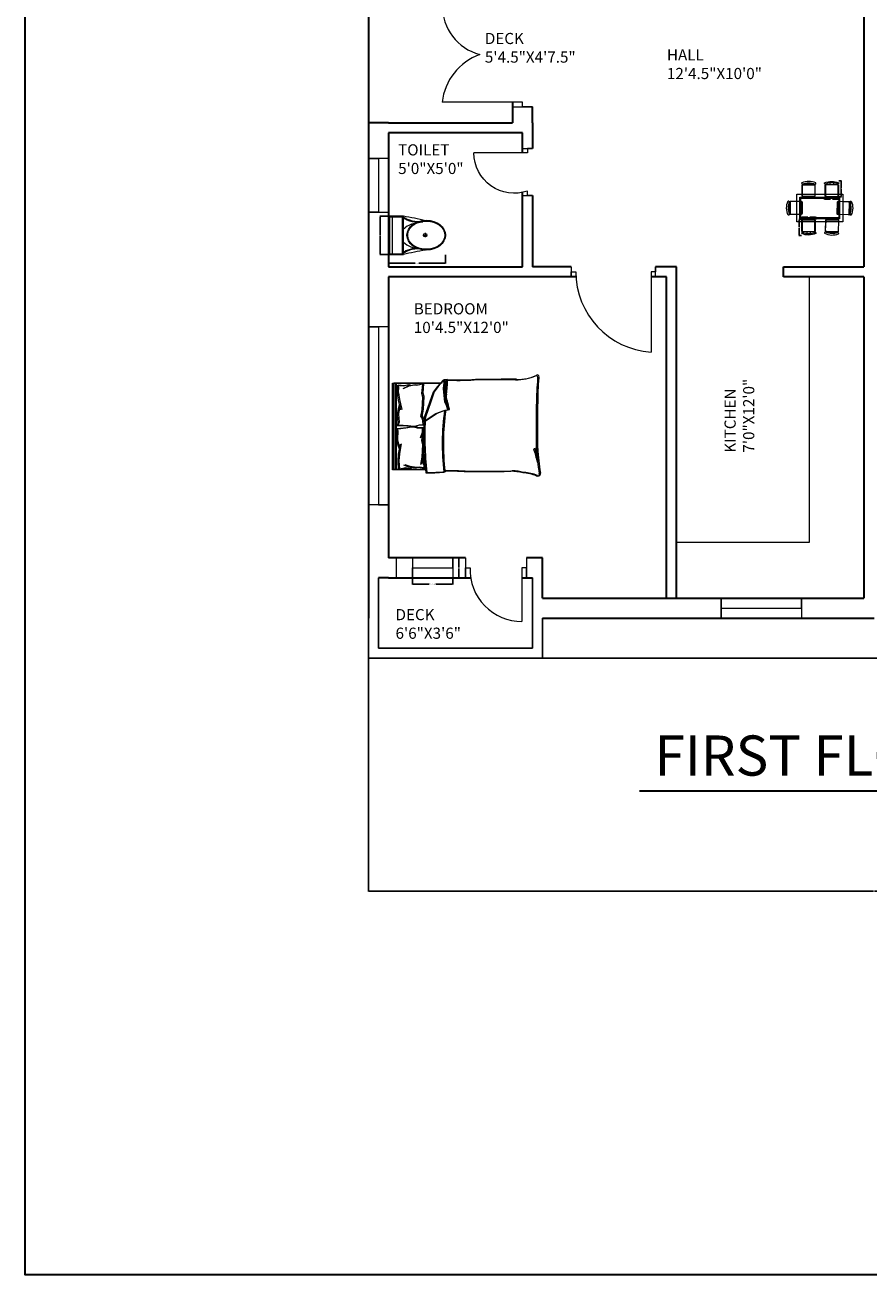
# Model space of a CAD drawing. Units: inches. Extents: x 2250 to 3629, y 982 to 2740.
# Tile 1 of 12: x 2250 to 2628, y 982 to 1543. Entities that reach past the tile are written whole.
import ezdxf

# ---------------------------------------------------------------- set-up
doc = ezdxf.new("R2010")
doc.units = ezdxf.units.IN
for name, color, linetype, lineweight in [('A-ANNO-DIMS', 2, 'Continuous', 18), ('A-ANNO-TITL', 7, 'Continuous', 35), ('A-ANNO-TTLB', 7, 'Continuous', 35), ('A-AREA-IDEN', 7, 'Continuous', 18), ('A-DOOR', 3, 'Continuous', 18), ('A-FLOR-DECK', 7, 'Continuous', 25), ('A-FLOR-FIXT', 9, 'Continuous', 18), ('A-FURN', 8, 'Continuous', 13), ('A-GLAZ', 4, 'Continuous', 18), ('A-WALL', 7, 'Continuous', 35)]:
    doc.layers.add(name, color=color, linetype=linetype, lineweight=lineweight)
doc.styles.get("Standard").update_dxf_attribs({"font": 'arial.ttf'})
doc.dimstyles.get("Standard").update_dxf_attribs({"dimtxt": 0.18, "dimasz": 0.18, "dimexe": 0.18, "dimexo": 0.0625, "dimgap": 0.09, "dimtad": 0, "dimtih": 1, "dimtoh": 1, "dimdec": 4, "dimzin": 0, "dimdsep": 46, "dimtxsty": 'Standard', "dimcen": 0.09, "dimadec": 0, "dimazin": 0, "dimtfac": 1, "dimtdec": 4, "dimtofl": 0, "dimtmove": 0, "dimatfit": 3, "dimfxl": 1, "dimtolj": 1, "dimtzin": 0, "dimarcsym": 0})

# ---------------------------------------------------------------- blocks, each defined once
blk = doc.blocks.new('A$C31115884')
for p, q in [((258, 466), (258, 523)), ((283, 498), (223, 498)), ((0, 200), (0, 0)), ((520, 200), (0, 200)), ((10, 190), (10, 10)), ((510, 190), (10, 190)), ((510, 10), (510, 190)), ((520, 0), (520, 200)), ((510, 54), (0, 54)), ((10, 10), (510, 10)), ((0, 0), (520, 0))]:
    blk.add_line(p, q)
blk.add_circle((256, 496), 23.6)
for centre, radius, start, end in [((2778, -205), 2807, 165.4549, 171.7133), ((-295, 403), 365, 324.2091, 9.3499), ((-295, 403), 375, 324.2091, 9.3499), ((384, 406), 293, 190.2774, 224.1564), ((139, 406), 293, 315.8436, 2.6563), ((806, 403), 375, 179.2036, 215.7909), ((806, 403), 365, 170.6501, 215.7909), ((3237, 905), 2807, 188.2867, 194.5451)]:
    blk.add_arc(centre, radius, start, end)
blk.add_ellipse((256, 510), major_axis=(0, -261), ratio=0.772727)
blk.add_open_spline([(256, 259), (263, 259), (270, 260), (288, 262), (299, 265), (320, 273), (330, 278), (350, 291), (360, 299), (378, 316), (386, 326), (402, 347), (409, 358), (421, 383), (427, 395), (436, 422), (440, 436), (445, 465), (447, 480), (448, 509), (448, 524), (445, 553), (443, 568), (436, 596), (432, 610), (422, 636), (416, 649), (402, 672), (395, 683), (379, 703), (370, 712), (351, 728), (341, 735), (321, 746), (310, 751), (289, 757), (278, 759), (256, 761), (245, 761), (223, 757), (212, 754), (191, 746), (181, 741), (161, 728), (151, 720), (133, 703), (125, 693), (110, 672), (103, 660), (90, 636), (85, 623), (76, 596), (72, 582), (67, 553), (66, 538), (64, 509), (65, 494), (68, 465), (70, 450), (77, 422), (81, 408), (91, 382), (97, 370), (111, 346), (118, 335), (135, 316), (144, 307), (162, 291), (172, 284), (193, 273), (203, 269), (225, 262), (236, 260), (250, 259), (253, 259), (256, 259)], degree=3, knots=[0, 0, 0, 0, 0.110105, 0.110105, 0.285049, 0.285049, 0.459994, 0.459994, 0.634938, 0.634938, 0.809882, 0.809882, 0.984827, 0.984827, 1.159771, 1.159771, 1.334715, 1.334715, 1.50966, 1.50966, 1.684604, 1.684604, 1.859549, 1.859549, 2.034493, 2.034493, 2.209437, 2.209437, 2.384382, 2.384382, 2.559326, 2.559326, 2.73427, 2.73427, 2.909215, 2.909215, 3.084159, 3.084159, 3.259103, 3.259103, 3.434048, 3.434048, 3.608992, 3.608992, 3.783936, 3.783936, 3.958881, 3.958881, 4.133825, 4.133825, 4.30877, 4.30877, 4.483714, 4.483714, 4.658658, 4.658658, 4.833603, 4.833603, 5.008547, 5.008547, 5.183491, 5.183491, 5.358436, 5.358436, 5.53338, 5.53338, 5.708324, 5.708324, 5.883269, 5.883269, 6.058213, 6.058213, 6.233158, 6.233158, 6.283185, 6.283185, 6.283185, 6.283185])
blk = doc.blocks.new('DR-24-BATH-SE')
for p, q in [((4.5, 21.1), (0, 21.1)), ((0, 21.1), (2.25, 21.1)), ((2.25, 21.1), (2.25, 19.1)), ((2.25, 19.1), (26.25, 19.1)), ((4.5, 0), (0, 0)), ((0, 0), (2.25, 0)), ((2.25, 0), (2.25, 2))]:
    blk.add_line(p, q)
blk.add_arc((8.16, 19.1), 18.09, 250.9415, 0)
blk = doc.blocks.new('DR-36-BED-SW')
for p, q in [((0, 38.25), (0, 33.75)), ((0, 33.75), (0, 36)), ((0, 36), (2, 36)), ((37.72, 36), (35.72, 36)), ((35.72, 36), (35.72, 0)), ((37.72, 33.75), (37.72, 38.25)), ((37.72, 38.25), (37.72, 36))]:
    blk.add_line(p, q)
blk.add_arc((38.08, 36), 36.08, 180, 266.2586)
blk = doc.blocks.new('DR-72-DECK-WEST-S')
for p, q in [((36, 45.46), (0, 45.46)), ((31.5, 47.46), (40.5, 47.46)), ((40.5, 47.46), (36, 47.46)), ((36, 47.46), (36, 45.46)), ((36, 2), (0, 2)), ((36, 0), (36, 2)), ((31.5, 0), (40.5, 0)), ((40.5, 0), (36, 0))]:
    blk.add_line(p, q)
for centre, radius, start, end in [((22.88, 45.46), 22.88, 180, 254.6216), ((25.61, -0.82), 25.77, 109.9642, 173.7115)]:
    blk.add_arc(centre, radius, start, end)
blk = doc.blocks.new('DR-24-DECK-SW')
for p, q in [((0, 28.5), (0, 19.5)), ((27.27, 28.5), (27.27, 19.5)), ((0, 19.5), (0, 24)), ((0, 24), (2, 24)), ((27.27, 24), (25.27, 24)), ((25.27, 24), (25.27, 0)), ((27.27, 19.5), (27.27, 24))]:
    blk.add_line(p, q)
blk.add_arc((25.27, 23.29), 23.29, 178.2408, 270)
blk = doc.blocks.new('WIN-24-DECK-NE')
for p, q in [((0, 4.5), (0, 9)), ((0, 9), (0, 0)), ((24, 0), (24, 9)), ((24, 9), (24, 4.5)), ((24, 4.5), (0, 4.5))]:
    blk.add_line(p, q)
blk = doc.blocks.new('WIN-36-KITCHEN-NE')
for p, q in [((0, 9), (0, 0)), ((0, 0), (0, 9)), ((0, 9), (0, 4.5)), ((36, 4.5), (36, 9)), ((36, 9), (36, 0)), ((0, 4.5), (36, 4.5))]:
    blk.add_line(p, q)
blk = doc.blocks.new('WIN-18-DECK-SW')
for p, q in [((0, 9), (0, 0)), ((18.04, 4.5), (18.04, 9)), ((18.04, 9), (18.04, 0)), ((0, 0), (0, 4.5)), ((0, 4.5), (18.04, 4.5))]:
    blk.add_line(p, q)
blk = doc.blocks.new('WIN-BED-SW')
for p, q in [((9, 79.76), (0, 79.76)), ((0, 79.76), (4.5, 79.76)), ((4.5, 79.76), (4.5, 0)), ((9, 0), (0, 0)), ((4.5, 0), (9, 0))]:
    blk.add_line(p, q)
blk = doc.blocks.new('BED-WITH-PILLOWS')
for p, q in [((2.83, 51.56), (2.83, 66.3)), ((2.83, 66.3), (41.74, 66.3)), ((2.83, 65.05), (41.74, 65.05)), ((3.02, 51.04), (3.02, 65.78)), ((3.02, 65.78), (41.92, 65.78)), ((3.02, 64.53), (41.92, 64.53)), ((3.17, 63.59), (6.66, 63.85)), ((3.17, 63.6), (3.64, 61.01)), ((3.36, 63.06), (6.85, 63.33)), ((3.36, 63.08), (3.83, 60.49)), ((6.66, 63.85), (6.75, 63.84)), ((6.75, 63.84), (9.86, 63.6)), ((6.85, 63.33), (6.93, 63.32)), ((6.93, 63.32), (10.04, 63.08)), ((9.86, 63.6), (14.33, 62.78)), ((10.04, 63.08), (14.52, 62.26)), ((12.09, 63.25), (13.74, 63.84)), ((12.28, 62.73), (13.93, 63.32)), ((13.74, 63.84), (16.09, 64.43)), ((13.93, 63.32), (16.28, 63.91)), ((16.09, 64.43), (16.36, 64.43)), ((16.28, 63.91), (16.54, 63.91)), ((16.36, 64.43), (19.98, 64.31)), ((16.54, 63.91), (20.16, 63.79)), ((19.98, 64.31), (21.15, 64.78)), ((20.16, 63.79), (21.34, 64.26)), ((21.15, 64.78), (21.62, 60.43)), ((21.34, 64.26), (21.81, 59.9)), ((22.78, 64.27), (22.58, 59.9)), ((22.96, 63.75), (22.76, 59.38)), ((23.98, 63.88), (22.78, 64.27)), ((24.17, 63.36), (22.96, 63.75)), ((27.59, 64.22), (23.98, 63.88)), ((27.77, 63.7), (24.17, 63.36)), ((27.85, 64.24), (27.59, 64.22)), ((28.03, 63.72), (27.77, 63.7)), ((30.23, 63.8), (27.85, 64.24)), ((30.42, 63.28), (28.03, 63.72)), ((34.12, 63.8), (29.71, 62.7)), ((34.31, 63.28), (29.9, 62.18)), ((31.91, 63.31), (30.23, 63.8)), ((32.1, 62.79), (30.42, 63.28)), ((37.22, 64.23), (34.12, 63.8)), ((37.4, 63.71), (34.31, 63.28)), ((40.8, 64.22), (36.4, 64.3)), ((36.4, 64.3), (37.22, 64.23)), ((40.98, 63.7), (36.58, 63.78)), ((36.58, 63.78), (37.4, 63.71)), ((40.14, 59.58), (39.18, 61.76)), ((40.8, 64.22), (40.49, 61.61)), ((40.98, 63.7), (40.67, 61.09)), ((41.74, 66.3), (41.74, 44.64)), ((41.92, 65.78), (41.92, 44.12)), ((3.64, 61.01), (3.29, 58.89)), ((3.29, 58.89), (3.76, 58.07)), ((3.83, 60.49), (3.47, 58.37)), ((3.47, 58.37), (3.95, 57.55)), ((3.64, 56.07), (4.11, 59.01)), ((3.88, 54.78), (3.64, 56.07)), ((3.83, 55.55), (4.3, 58.49)), ((4.11, 59.01), (4.94, 61.25)), ((4.3, 58.49), (5.12, 60.73)), ((21.62, 60.43), (22.09, 57.84)), ((22.09, 56.78), (21.62, 55.25)), ((21.81, 59.9), (22.28, 57.32)), ((22.28, 56.26), (21.81, 54.73)), ((22.09, 57.84), (22.09, 56.78)), ((22.58, 59.9), (22.27, 57.28)), ((22.27, 57.28), (22.34, 56.23)), ((22.28, 57.32), (22.28, 56.26)), ((22.34, 56.23), (22.9, 54.73)), ((22.76, 59.38), (22.46, 56.76)), ((22.46, 56.76), (22.52, 55.71)), ((40.33, 59.06), (39.37, 61.24)), ((40.8, 56.67), (40.14, 59.58)), ((40.98, 56.15), (40.33, 59.06)), ((40.49, 61.61), (40.97, 59.51)), ((40.97, 59.51), (40.55, 58.66)), ((40.64, 55.37), (40.8, 56.67)), ((40.67, 61.09), (41.16, 58.99)), ((41.16, 58.99), (40.74, 58.14)), ((40.83, 54.85), (40.98, 56.15)), ((3.41, 52.19), (3.88, 54.78)), ((7.56, 52.77), (3.41, 52.19)), ((3.59, 51.66), (4.06, 54.25)), ((7.74, 52.25), (3.59, 51.66)), ((4.06, 54.25), (3.83, 55.55)), ((5.2, 53.58), (8.48, 53.04)), ((5.38, 53.06), (8.66, 52.52)), ((8.48, 53.04), (7.56, 52.77)), ((8.66, 52.52), (7.74, 52.25)), ((8.48, 53.04), (14.18, 52.69)), ((8.66, 52.52), (14.37, 52.17)), ((14.18, 52.69), (15.78, 53.14)), ((14.37, 52.17), (15.97, 52.62)), ((15.78, 53.14), (19.96, 52.81)), ((15.97, 52.62), (20.14, 52.29)), ((19.62, 53.06), (17.06, 53.95)), ((19.81, 52.54), (17.25, 53.43)), ((21.62, 53.06), (19.62, 53.06)), ((21.81, 52.54), (19.81, 52.54)), ((21.62, 55.25), (21.62, 53.06)), ((21.81, 54.73), (21.81, 52.54)), ((22.52, 55.71), (23.09, 54.21)), ((22.9, 54.73), (23.04, 52.55)), ((23.04, 52.55), (25.03, 52.68)), ((23.09, 54.21), (23.22, 52.03)), ((23.22, 52.03), (25.22, 52.15)), ((24.63, 52.15), (28.05, 46.86)), ((24.82, 51.63), (28.23, 46.34)), ((25.03, 52.68), (27.53, 53.72)), ((25.22, 52.15), (27.72, 53.2)), ((33.09, 49.76), (26.3, 52.15)), ((33.27, 49.24), (26.49, 51.63)), ((26.51, 53.58), (29.79, 53.04)), ((26.7, 53.06), (29.98, 52.52)), ((29.79, 53.04), (35.5, 52.69)), ((29.98, 52.52), (35.69, 52.17)), ((35.5, 52.69), (37.1, 53.14)), ((35.69, 52.17), (37.28, 52.62)), ((37.1, 53.14), (41.27, 52.81)), ((37.28, 52.62), (41.46, 52.29)), ((41.27, 52.81), (40.64, 55.37)), ((41.46, 52.29), (40.83, 54.85)), ((28.05, 46.86), (29.43, 43.21)), ((28.23, 46.34), (29.62, 42.69)), ((37.63, 48.12), (33.09, 49.76)), ((37.81, 47.6), (33.27, 49.24)), ((40.02, 46.36), (37.63, 48.12)), ((40.21, 45.84), (37.81, 47.6)), ((43.04, 43.71), (40.02, 46.36)), ((43.23, 43.19), (40.21, 45.84)), ((29.43, 43.21), (29.68, 41.57)), ((29.62, 42.69), (29.87, 41.05)), ((29.68, 41.57), (31.7, 42.08)), ((29.87, 41.05), (31.89, 41.56)), ((31.7, 42.08), (33.34, 42.83)), ((31.89, 41.56), (33.53, 42.31)), ((33.34, 42.83), (36.11, 43.21)), ((33.53, 42.31), (36.3, 42.69)), ((36.11, 43.21), (39.27, 43.46)), ((36.3, 42.69), (39.45, 42.94)), ((39.27, 43.46), (41.79, 43.21)), ((39.45, 42.94), (41.97, 42.69)), ((41.79, 43.21), (43.04, 43.71)), ((41.97, 42.69), (43.23, 43.19)), ((43.1, 42.29), (43.04, 43.71, 3.15)), ((43.29, 41.77), (43.23, 43.19, 3.15)), ((12.26, 1.79), (32.3, 1.79)), ((12.45, 1.27), (32.49, 1.27))]:
    blk.add_line(p, q)
for centre, radius, start, end in [((69.33, 49.94), 67.82, 178.7218, 185.604), ((17.39, -81.91), 134.3, 86.0865, 96.7821), ((69.52, 49.42), 67.82, 178.7218, 185.604), ((17.57, -82.43), 134.3, 86.0865, 96.7821), ((14.46, -60.96), 105.04, 81.7845, 96.9006), ((14.64, -61.48), 105.04, 81.7845, 96.9006), ((-136.21, 40.92), 138.49, 358.4762, 1.0082), ((-136.02, 40.4), 138.49, 358.4762, 1.0082), ((29.83, 41.52), 0.15, 160.2464, 271.1377), ((25.36, 65.1), 24.14, 280.6617, 289.8806), ((30.01, 41), 0.15, 160.2464, 271.1377), ((25.55, 64.58), 24.14, 280.6617, 289.8806), ((35.61, 37.76), 5.07, 78.6608, 113.7384), ((35.8, 37.23), 5.07, 78.6608, 113.7384), ((41.79, 71.72), 29.46, 259.8763, 272.5657), ((41.97, 71.2), 29.46, 259.8763, 272.5657), ((148.38, 36.74), 105.43, 176.9791, 183.8365), ((148.57, 36.22), 105.43, 176.9791, 183.8365), ((394.7, 25.1), 392.65, 178.2277, 181.7185), ((394.88, 24.58), 392.65, 178.2277, 181.7185), ((-3670.6, 11.09), 3713.84, 0.00217, 0.28689), ((-3670.41, 10.57), 3713.84, 0.00217, 0.28689), ((-21.9, 13.78), 24.13, 346.0648, 358.9113), ((-21.71, 13.26), 24.13, 346.0648, 358.9113), ((62, 10.4), 18.78, 177.4714, 206.4681), ((-17.63, 9.09), 19.18, 337.9751, 356.652), ((-17.45, 8.57), 19.18, 337.9751, 356.652), ((62.19, 9.88), 18.78, 177.4714, 206.4681), ((0.89, 1.4), 0.887, 146.1736, 293.4781), ((1.07, 0.88), 0.887, 146.1736, 293.4781), ((17.44, -97.2), 99.12, 92.9958, 99.4091), ((17.63, -97.72), 99.12, 92.9958, 99.4091), ((-14.02, 85.61), 86.67, 283.3832, 287.7053), ((-13.83, 85.09), 86.67, 283.3832, 287.7053), ((33.5, -106.51), 108.31, 84.4998, 90.6351), ((33.69, -107.03), 108.31, 84.4998, 90.6351), ((44.3, 2.09), 0.897, 242.6588, 356.02), ((44.48, 1.57), 0.897, 242.6588, 356.02)]:
    blk.add_arc(centre, radius, start, end)
blk = doc.blocks.new('CHAIR-DINING-2')
for points in [[(0.44, 5.7, -0.578392), (0.02, 6.17, -0.214524), (6.35, 6.26, -0.552014), (6.06, 5.75, 0.175809), (0.44, 5.7)], [(2.51, 5.52), (2.51, 6.18, 0.064759)], [(5.89, 5.52, -0.414214), (6.26, 5.16), (6.26, 0.36, -0.414214), (5.89, 0), (0.68, 0, -0.414214), (0.32, 0.36), (0.32, 5.16, -0.414214), (0.68, 5.52), (5.89, 5.52)]]:
    blk.add_lwpolyline(points, format="xyb")
blk.add_lwpolyline([(3.97, 6.19), (3.97, 5.52)])
blk.add_lwpolyline([(5.89, 5.36), (0.84, 5.36, 0.414214), (0.48, 4.99), (0.48, 0.53, 0.414214), (0.84, 0.16), (5.89, 0.16, 0.512069), (6.09, 0.53), (6.09, 4.99, 0.512069)], format="xyb", close=True)
blk = doc.blocks.new('CHAIR-DINING-5')
for points in [[(5.71, 1.37), (0.5, 1.37, -0.414214), (0.14, 1.74), (0.14, 6.53, -0.414214), (0.5, 6.89), (5.71, 6.89, -0.414214), (6.08, 6.53), (6.08, 1.74, -0.414214), (5.71, 1.37)], [(5.95, 1.19, -0.578392), (6.38, 0.72, -0.214524), (0.04, 0.64, -0.552014), (0.34, 1.15, 0.175809), (5.95, 1.19)], [(3.88, 1.37), (3.88, 0.71, 0.064759)]]:
    blk.add_lwpolyline(points, format="xyb")
blk.add_lwpolyline([(0.5, 1.54), (5.55, 1.54, 0.414214), (5.91, 1.9), (5.91, 6.37, 0.414214), (5.55, 6.73), (0.5, 6.73, 0.512069), (0.3, 6.37), (0.3, 1.9, 0.512069)], format="xyb", close=True)
blk.add_lwpolyline([(2.42, 0.7), (2.42, 1.37)])
blk = doc.blocks.new('TABLE-RECTANGULAR')
for points in [[(0, 12.37), (20.61, 12.37), (20.61, 0), (0, 0)], [(1.37, 10.99), (19.24, 10.99), (19.24, 1.37), (1.37, 1.37)], [(1.79, 10.58), (18.82, 10.58), (18.82, 1.79), (1.79, 1.79)]]:
    blk.add_lwpolyline(points, close=True)
blk = doc.blocks.new('*D59')
at = {"layer": 'A-ANNO-DIMS', "color": 0, "lineweight": -2, "transparency": 16777216}
for p, q in [((2412.61, 1439.61), (2412.61, 1435.67)), ((2412.79, 1435.85), (2424.57, 1435.85)), ((2437.91, 1435.85), (2426.12, 1435.85)), ((2438.09, 1439.61), (2438.09, 1435.67))]:
    blk.add_line(p, q, dxfattribs=at)
at = {"layer": 'A-ANNO-DIMS', "color": 0, "transparency": 16777216}
for points in [[(2412.79, 1435.88), (2412.79, 1435.82), (2412.61, 1435.85)], [(2437.91, 1435.88), (2437.91, 1435.82), (2438.09, 1435.85)]]:
    blk.add_solid(points, dxfattribs=at)
at = {"layer": 'Defpoints', "color": 0, "transparency": 16777216}
for p in [(2412.61, 1439.68), (2438.09, 1439.68), (2438.09, 1435.85)]:
    blk.add_point(p, dxfattribs=at)
at = {"layer": 'A-ANNO-DIMS', "color": 0, "transparency": 16777216, "insert": (2425.35, 1435.85), "char_height": 0.18, "attachment_point": 5}
blk.add_mtext('\\A1;WC 25 TYP.', dxfattribs=at)
blk = doc.blocks.new('*D60')
at = {"layer": 'A-ANNO-DIMS', "color": 0, "lineweight": -2, "transparency": 16777216}
for p, q in [((2412.54, 1456.87), (2408.61, 1456.87)), ((2408.79, 1456.69), (2408.79, 1448.45)), ((2408.79, 1439.86), (2408.79, 1448.09)), ((2412.54, 1439.68), (2408.61, 1439.68))]:
    blk.add_line(p, q, dxfattribs=at)
at = {"layer": 'A-ANNO-DIMS', "color": 0, "transparency": 16777216}
for points in [[(2408.76, 1456.69), (2408.82, 1456.69), (2408.79, 1456.87)], [(2408.76, 1439.86), (2408.82, 1439.86), (2408.79, 1439.68)]]:
    blk.add_solid(points, dxfattribs=at)
at = {"layer": 'Defpoints', "color": 0, "transparency": 16777216}
for p in [(2412.61, 1456.87), (2408.79, 1439.68), (2412.61, 1439.68)]:
    blk.add_point(p, dxfattribs=at)
at = {"layer": 'A-ANNO-DIMS', "color": 0, "transparency": 16777216, "insert": (2408.79, 1448.27), "char_height": 0.18, "attachment_point": 5}
blk.add_mtext('\\A1;17 TYP.', dxfattribs=at)
blk = doc.blocks.new('*D67')
at = {"layer": 'A-ANNO-DIMS', "color": 0, "lineweight": -2, "transparency": 16777216}
for p, q in [((2614.39, 1472.75), (2615.58, 1472.75)), ((2615.4, 1472.57), (2615.4, 1469.37)), ((2615.4, 1465.8), (2615.4, 1469)), ((2614.39, 1465.62), (2615.58, 1465.62))]:
    blk.add_line(p, q, dxfattribs=at)
at = {"layer": 'A-ANNO-DIMS', "color": 0, "transparency": 16777216}
for points in [[(2615.37, 1472.57), (2615.43, 1472.57), (2615.4, 1472.75)], [(2615.37, 1465.8), (2615.43, 1465.8), (2615.4, 1465.62)]]:
    blk.add_solid(points, dxfattribs=at)
at = {"layer": 'Defpoints', "color": 0, "transparency": 16777216}
for p in [(2614.33, 1472.75), (2615.4, 1472.75), (2614.33, 1465.62)]:
    blk.add_point(p, dxfattribs=at)
at = {"layer": 'A-ANNO-DIMS', "color": 0, "transparency": 16777216, "insert": (2615.4, 1469.19), "char_height": 0.18, "attachment_point": 5}
blk.add_mtext('\\A1;CHAIR B 7 TYP.', dxfattribs=at)
blk = doc.blocks.new('*D68')
at = {"layer": 'A-ANNO-DIMS', "color": 0, "lineweight": -2, "transparency": 16777216}
for p, q in [((2607.9, 1465.56), (2607.9, 1464.37)), ((2608.08, 1464.55), (2610.66, 1464.55)), ((2614.15, 1464.55), (2611.57, 1464.55)), ((2614.33, 1465.56), (2614.33, 1464.37))]:
    blk.add_line(p, q, dxfattribs=at)
at = {"layer": 'A-ANNO-DIMS', "color": 0, "transparency": 16777216}
for points in [[(2608.08, 1464.58), (2608.08, 1464.52), (2607.9, 1464.55)], [(2614.15, 1464.58), (2614.15, 1464.52), (2614.33, 1464.55)]]:
    blk.add_solid(points, dxfattribs=at)
at = {"layer": 'Defpoints', "color": 0, "transparency": 16777216}
for p in [(2607.9, 1465.62), (2614.33, 1465.62), (2614.33, 1464.55)]:
    blk.add_point(p, dxfattribs=at)
at = {"layer": 'A-ANNO-DIMS', "color": 0, "transparency": 16777216, "insert": (2611.12, 1464.55), "char_height": 0.18, "attachment_point": 5}
blk.add_mtext('\\A1;6 TYP.', dxfattribs=at)
blk = doc.blocks.new('*D69')
at = {"layer": 'A-ANNO-DIMS', "color": 0, "lineweight": -2, "transparency": 16777216}
for p, q in [((2597.61, 1455.36), (2596.42, 1455.36)), ((2596.6, 1455.18), (2596.6, 1451.97)), ((2596.6, 1448.4), (2596.6, 1451.61)), ((2597.61, 1448.22), (2596.42, 1448.22))]:
    blk.add_line(p, q, dxfattribs=at)
at = {"layer": 'A-ANNO-DIMS', "color": 0, "transparency": 16777216}
for points in [[(2596.57, 1455.18), (2596.63, 1455.18), (2596.6, 1455.36)], [(2596.57, 1448.4), (2596.63, 1448.4), (2596.6, 1448.22)]]:
    blk.add_solid(points, dxfattribs=at)
at = {"layer": 'Defpoints', "color": 0, "transparency": 16777216}
for p in [(2596.6, 1455.36), (2597.67, 1455.36), (2597.67, 1448.22)]:
    blk.add_point(p, dxfattribs=at)
at = {"layer": 'A-ANNO-DIMS', "color": 0, "transparency": 16777216, "insert": (2596.6, 1451.79), "char_height": 0.18, "attachment_point": 5}
blk.add_mtext('\\A1;CHAIR C 7 TYP.', dxfattribs=at)
blk = doc.blocks.new('*D70')
at = {"layer": 'A-ANNO-DIMS', "color": 0, "lineweight": -2, "transparency": 16777216}
for p, q in [((2597.67, 1455.42), (2597.67, 1456.61)), ((2597.85, 1456.43), (2600.43, 1456.43)), ((2603.92, 1456.43), (2601.35, 1456.43)), ((2604.1, 1455.42), (2604.1, 1456.61))]:
    blk.add_line(p, q, dxfattribs=at)
at = {"layer": 'A-ANNO-DIMS', "color": 0, "transparency": 16777216}
for points in [[(2597.85, 1456.46), (2597.85, 1456.4), (2597.67, 1456.43)], [(2603.92, 1456.46), (2603.92, 1456.4), (2604.1, 1456.43)]]:
    blk.add_solid(points, dxfattribs=at)
at = {"layer": 'Defpoints', "color": 0, "transparency": 16777216}
for p in [(2597.67, 1455.36), (2604.1, 1456.43), (2604.1, 1455.36)]:
    blk.add_point(p, dxfattribs=at)
at = {"layer": 'A-ANNO-DIMS', "color": 0, "transparency": 16777216, "insert": (2600.89, 1456.43), "char_height": 0.18, "attachment_point": 5}
blk.add_mtext('\\A1;6 TYP.', dxfattribs=at)
blk = doc.blocks.new('*D81')
at = {"layer": 'A-ANNO-DIMS', "color": 0, "lineweight": -2, "transparency": 16777216}
for p, q in [((2423.28, 1294.67), (2423.28, 1291.85)), ((2441.33, 1294.67), (2441.33, 1291.85)), ((2423.46, 1292.03), (2430.81, 1292.03)), ((2441.15, 1292.03), (2433.8, 1292.03))]:
    blk.add_line(p, q, dxfattribs=at)
at = {"layer": 'A-ANNO-DIMS', "color": 0, "transparency": 16777216}
for points in [[(2423.46, 1292.06), (2423.46, 1292), (2423.28, 1292.03)], [(2441.15, 1292.06), (2441.15, 1292), (2441.33, 1292.03)]]:
    blk.add_solid(points, dxfattribs=at)
at = {"layer": 'Defpoints', "color": 0, "transparency": 16777216}
for p in [(2423.28, 1294.74), (2441.33, 1294.74), (2441.33, 1292.03)]:
    blk.add_point(p, dxfattribs=at)
at = {"layer": 'A-ANNO-DIMS', "color": 0, "transparency": 16777216, "insert": (2432.3, 1292.03), "char_height": 0.18, "attachment_point": 5}
blk.add_mtext('\\A1;DECK WINDOW 18 TYP.', dxfattribs=at)
blk = doc.blocks.new('*D82')
at = {"layer": 'A-ANNO-DIMS', "color": 0, "lineweight": -2, "transparency": 16777216}
for p, q in [((2441.39, 1303.74), (2444.21, 1303.74)), ((2444.03, 1303.56), (2444.03, 1299.42)), ((2441.39, 1294.74), (2444.21, 1294.74)), ((2444.03, 1294.92), (2444.03, 1299.05))]:
    blk.add_line(p, q, dxfattribs=at)
at = {"layer": 'A-ANNO-DIMS', "color": 0, "transparency": 16777216}
for points in [[(2444, 1303.56), (2444.06, 1303.56), (2444.03, 1303.74)], [(2444, 1294.92), (2444.06, 1294.92), (2444.03, 1294.74)]]:
    blk.add_solid(points, dxfattribs=at)
at = {"layer": 'Defpoints', "color": 0, "transparency": 16777216}
for p in [(2441.33, 1303.74), (2444.03, 1303.74), (2441.33, 1294.74)]:
    blk.add_point(p, dxfattribs=at)
at = {"layer": 'A-ANNO-DIMS', "color": 0, "transparency": 16777216, "insert": (2444.03, 1299.24), "char_height": 0.18, "attachment_point": 5}
blk.add_mtext('\\A1;9 TYP.', dxfattribs=at)
blk = doc.blocks.new('*D169')
at = {"layer": 'A-ANNO-DIMS', "color": 0, "lineweight": -2, "transparency": 16777216}
for p, q in [((2856.61, 1276.67), (2856.61, 1154.23)), ((2403.61, 1258.67), (2403.61, 1154.23)), ((2403.79, 1154.41), (2629.81, 1154.41)), ((2856.43, 1154.41), (2630.4, 1154.41))]:
    blk.add_line(p, q, dxfattribs=at)
at = {"layer": 'A-ANNO-DIMS', "color": 0, "transparency": 16777216}
for points in [[(2403.79, 1154.44), (2403.79, 1154.38), (2403.61, 1154.41)], [(2856.43, 1154.44), (2856.43, 1154.38), (2856.61, 1154.41)]]:
    blk.add_solid(points, dxfattribs=at)
at = {"layer": 'Defpoints', "color": 0, "transparency": 16777216}
for p in [(2856.61, 1276.74), (2403.61, 1258.74), (2856.61, 1154.41)]:
    blk.add_point(p, dxfattribs=at)
at = {"layer": 'A-ANNO-DIMS', "color": 0, "transparency": 16777216, "insert": (2630.11, 1154.41), "char_height": 0.18, "attachment_point": 5}
blk.add_mtext('\\A1;453', dxfattribs=at)
blk = doc.blocks.new('*D170')
at = {"layer": 'A-ANNO-DIMS', "color": 0, "lineweight": -2, "transparency": 16777216}
for p, q in [((2855.4, 2070.24), (2901.69, 2070.24)), ((2901.51, 2070.06), (2901.51, 1664.67)), ((2901.51, 1258.92), (2901.51, 1664.3)), ((2481.67, 1258.74), (2901.69, 1258.74))]:
    blk.add_line(p, q, dxfattribs=at)
at = {"layer": 'A-ANNO-DIMS', "color": 0, "transparency": 16777216}
for points in [[(2901.48, 2070.06), (2901.54, 2070.06), (2901.51, 2070.24)], [(2901.48, 1258.92), (2901.54, 1258.92), (2901.51, 1258.74)]]:
    blk.add_solid(points, dxfattribs=at)
at = {"layer": 'Defpoints', "color": 0, "transparency": 16777216}
for p in [(2855.34, 2070.24), (2901.51, 2070.24), (2481.61, 1258.74)]:
    blk.add_point(p, dxfattribs=at)
at = {"layer": 'A-ANNO-DIMS', "color": 0, "transparency": 16777216, "insert": (2901.51, 1664.49), "char_height": 0.18, "attachment_point": 5}
blk.add_mtext('\\A1;811.5', dxfattribs=at)

msp = doc.modelspace()

# ---------------------------------------------------------------- linework, layer by layer
at = {"layer": 'A-ANNO-TITL'}
msp.add_line((2524.9884, 1199.312), (2775.3748, 1199.312), dxfattribs=at)
at = {"layer": 'A-ANNO-TTLB'}
msp.add_lwpolyline([(2249.6849, 2739.593), (3629.4532, 2739.593), (3629.4532, 982.3108), (2249.6849, 982.3108)], close=True, dxfattribs=at)
at = {"layer": 'A-FLOR-DECK'}
for p, q in [((2408.1072, 1294.7354), (2408.1072, 1263.2354)), ((2477.1072, 1294.7354), (2477.1072, 1276.7354)), ((2403.6072, 1258.7354), (2403.6072, 1276.7354)), ((2477.1072, 1263.2354), (2477.1072, 1276.7354)), ((2481.6072, 1276.7354), (2481.6072, 1258.7354)), ((2408.1072, 1263.2354), (2477.1072, 1263.2354)), ((2481.6072, 1258.7354), (2403.6072, 1258.7354))]:
    msp.add_line(p, q, dxfattribs=at)
at = {"layer": 'A-FLOR-FIXT'}
for p, q in [((2600.9947, 1429.7354), (2600.9947, 1310.6354)), ((2600.9947, 1310.6354), (2541.6072, 1310.6354))]:
    msp.add_line(p, q, dxfattribs=at)
at = {"layer": 'A-FURN'}
for points in [[(2598.0256, 1471.3648, -0.17580919), (2603.6393, 1471.3223, 0.57839206), (2604.0646, 1471.7899, 0.21452438), (2597.7279, 1471.875, 0.55201397), (2598.0256, 1471.3648, -0.06507904)], [(2603.4012, 1471.1395), (2598.1896, 1471.1395, 0.41421356), (2597.825, 1470.7749), (2597.825, 1465.9829, 0.41421356), (2598.1896, 1465.6183), (2603.4012, 1465.6183, 0.41421356), (2603.7658, 1465.9829), (2603.7658, 1470.7749, 0.41421356), (2603.4012, 1471.1395)], [(2601.5706, 1471.1395), (2601.5706, 1471.7986, -0.06475861)], [(2592.1526, 1457.8085, -0.57839206), (2591.6849, 1457.3832, -0.21452438), (2591.5999, 1463.7199, -0.55201397), (2592.11, 1463.4222, 0.17580937), (2592.1526, 1457.8085)], [(2592.3354, 1463.2583, -0.41421356), (2592.7, 1463.6229), (2597.4919, 1463.6229, -0.41421356), (2597.8565, 1463.2583), (2597.8565, 1458.0467, -0.41421356), (2597.4919, 1457.6821), (2592.7, 1457.6821, -0.41421356), (2592.3354, 1458.0467), (2592.3354, 1463.2583)], [(2592.3354, 1459.8772), (2591.6762, 1459.8772, 0.06475861)]]:
    msp.add_lwpolyline(points, format="xyb", dxfattribs=at)
for points in [[(2598.1918, 1470.9752), (2603.2369, 1470.9752, -0.41421356), (2603.6015, 1470.6106), (2603.6015, 1466.1472, -0.41421356), (2603.2369, 1465.7826), (2598.1918, 1465.7826, -0.51206948), (2597.9892, 1466.1472), (2597.9892, 1470.6106, -0.51206948)], [(2592.4996, 1463.2561), (2592.4996, 1458.2109, 0.41421356), (2592.8642, 1457.8463), (2597.3277, 1457.8463, 0.41421356), (2597.6923, 1458.2109), (2597.6923, 1463.2561, 0.51206948), (2597.3277, 1463.4586), (2592.8642, 1463.4586, 0.51206948)]]:
    msp.add_lwpolyline(points, format="xyb", close=True, dxfattribs=at)
for points in [[(2600.1118, 1471.8106), (2600.1118, 1471.1395)], [(2591.6643, 1461.336), (2592.3354, 1461.336)]]:
    msp.add_lwpolyline(points, dxfattribs=at)
at = {"layer": 'A-GLAZ'}
msp.add_line((2415.987, 1303.7354), (2415.987, 1294.7354), dxfattribs=at)
at = {"layer": 'A-WALL'}
for p, q in [((2403.6072, 2047.7354), (2403.6072, 1276.7354)), ((2625.6072, 1638.2354), (2625.6072, 1434.2354)), ((2468.1072, 1507.9638), (2468.1072, 1498.7354)), ((2477.1072, 1498.7354), (2477.1072, 1505.9638)), ((2412.6072, 1498.7354), (2403.6072, 1498.7354)), ((2412.6072, 1498.7354), (2468.1072, 1498.7354)), ((2477.1072, 1498.7354), (2477.1072, 1487.263)), ((2472.6072, 1494.2354), (2412.6072, 1494.2354)), ((2412.6072, 1494.2354), (2412.6072, 1434.2354)), ((2472.6072, 1485.263), (2472.6072, 1494.2354)), ((2472.6072, 1434.2354), (2472.6072, 1467.5923)), ((2477.1072, 1466.2174), (2477.1072, 1434.2354)), ((2412.6072, 1434.2354), (2472.6072, 1434.2354)), ((2496.5413, 1429.7354), (2412.6072, 1429.7354)), ((2412.6072, 1429.7354), (2412.6072, 1303.7354)), ((2494.4711, 1434.2354), (2477.1072, 1434.2354)), ((2537.1072, 1429.7354), (2530.1938, 1429.7354)), ((2541.6072, 1434.2354), (2532.1938, 1434.2354)), ((2537.1072, 1405.7354), (2537.1072, 1429.7354)), ((2541.6072, 1285.7354), (2541.6072, 1434.2354)), ((2589.6246, 1434.2354), (2625.6072, 1434.2354)), ((2589.6246, 1429.7354), (2589.6246, 1434.2354)), ((2625.6072, 1429.7354), (2589.6246, 1429.7354)), ((2625.6072, 1429.7354), (2625.6072, 1285.7354)), ((2537.1072, 1285.7354), (2537.1072, 1405.7354)), ((2447.1072, 1303.7354), (2412.6072, 1303.7354)), ((2481.6072, 1303.7354), (2474.3814, 1303.7354)), ((2481.6072, 1285.7354), (2481.6072, 1303.7354)), ((2412.6072, 1294.7354), (2408.1072, 1294.7354)), ((2412.6072, 1294.7354), (2449.4059, 1294.7354)), ((2472.3814, 1294.7354), (2477.1072, 1294.7354)), ((2481.6072, 1285.7354), (2537.1072, 1285.7354)), ((2481.6072, 1285.7354), (2625.6072, 1285.7354)), ((2537.1072, 1285.7354), (2541.6072, 1285.7354)), ((2481.6072, 1276.7354), (2630.1072, 1276.7354))]:
    msp.add_line(p, q, dxfattribs=at)

# ---------------------------------------------------------------- block references
at = {"layer": 'A-DOOR'}
for name, p in [('DR-72-DECK-WEST-S', (2436.607, 1505.964)), ('DR-36-BED-SW', (2494.471, 1395.985)), ('DR-24-DECK-SW', (2447.107, 1275.235))]:
    msp.add_blockref(name, p, dxfattribs=at)
at = {"layer": 'A-DOOR', "extrusion": (0, 0, -1), "zscale": -1, "rotation": 359.9465721628409}
msp.add_blockref('DR-24-BATH-SE', (-2477.1164, 1466.1894), dxfattribs=at)
at = {"layer": 'A-FLOR-FIXT', "xscale": 0.0330640103915726, "yscale": 0.0330640103915726, "zscale": 0.0330640103915726, "rotation": 269.9999999999999}
msp.add_blockref('A$C31115884', (2412.6072, 1456.8683), dxfattribs=at)
at = {"layer": 'A-FURN'}
for name, p in [('CHAIR-DINING-2', (2607.923, 1465.618)), ('TABLE-RECTANGULAR', (2595.4765, 1454.3714)), ('CHAIR-DINING-5', (2597.688, 1448.465))]:
    msp.add_blockref(name, p, dxfattribs=at)
for name, p, rotation in [('CHAIR-DINING-2', (2613.7796, 1463.9335), 267.811102945421), ('BED-WITH-PILLOWS', (2480.6933, 1340.361), 89.99999999999999)]:
    msp.add_blockref(name, p, dxfattribs=dict(at, rotation=rotation))
at = {"layer": 'A-FURN', "extrusion": (0, 0, -1), "zscale": -1, "rotation": 2.165162275592024}
msp.add_blockref('CHAIR-DINING-5', (-2614.2684, 1448.3533), dxfattribs=at)
at = {"layer": 'A-GLAZ', "rotation": 90.0000000000001}
msp.add_blockref('WIN-24-DECK-NE', (2412.6076, 1458.7153), dxfattribs=at)
at = {"layer": 'A-GLAZ'}
for name, p in [('WIN-BED-SW', (2403.607, 1327.592)), ('WIN-18-DECK-SW', (2423.282, 1294.735)), ('WIN-36-KITCHEN-NE', (2561.6893, 1276.735))]:
    msp.add_blockref(name, p, dxfattribs=at)

# ---------------------------------------------------------------- texts
at = {"layer": 'A-ANNO-TITL', "insert": (2531.7555, 1224.1419), "char_height": 18, "attachment_point": 1}
msp.add_mtext_dynamic_manual_height_columns('FIRST FLOOR PLAN', width=297.220022, gutter_width=12.5, heights=[0], dxfattribs=at)
at = {"layer": 'A-AREA-IDEN', "char_height": 5, "attachment_point": 1}
for s, width, insert in [('DECK\\P5\'4.5"X4\'7.5"', 63.091736, (2455.7433, 1539.0614)), ('HALL\\P12\'4.5"X10\'0"', 146.389302, (2537.3237, 1531.7037)), ('TOILET\\P5\'0"X5\'0"', 82.224606, (2416.8853, 1489.1373)), ('BEDROOM\\P10\'4.5"X12\'0"', 99.309214, (2423.9036, 1417.8903)), ('DECK\\P6\'6"X3\'6"', 96.606177, (2415.7146, 1280.8151))]:
    msp.add_mtext_dynamic_manual_height_columns(s, width=width, gutter_width=12.5, heights=[0], dxfattribs=dict(at, insert=insert))
at = {"layer": 'A-AREA-IDEN', "insert": (2563.1317, 1350.9213), "char_height": 5, "attachment_point": 1, "rotation": 90}
msp.add_mtext_dynamic_manual_height_columns('KITCHEN\\P7\'0"X12\'0"', width=103.349357, gutter_width=12.5, heights=[0], dxfattribs=at)

# ---------------------------------------------------------------- dimensions: what is measured, and where the dimension line sits
at = {"layer": 'A-ANNO-DIMS'}
dim = msp.add_linear_dim(base=(2901.5072, 2070.2354), p1=(2481.6072, 1258.7354), p2=(2855.3384, 2070.2354), angle=90, dimstyle='Standard', override={"dimdec": 1, "dimlfac": 1, "dimrnd": 0, "dimzin": 0, "dimdsep": 46, "dimlunit": 2}, dxfattribs=at)
dim.commit()
dim.dimension.update_dxf_attribs({"geometry": '*D170', "text_midpoint": (2901.5072, 1664.4854)})
for base, p1, p2, angle, text, picture, middle in [((2615.4026, 1472.7542), (2614.3322, 1465.6183), (2614.3322, 1472.7542), 90, 'CHAIR B <> TYP.', '*D67', (2615.4026, 1469.1862)), ((2408.7855, 1439.675), (2412.6072, 1456.8683), (2412.6072, 1439.675), 270, '<> TYP.', '*D60', (2408.7855, 1448.2717)), ((2596.6021, 1455.3592), (2597.6725, 1448.2234), (2597.6725, 1455.3592), 90, 'CHAIR C <> TYP.', '*D69', (2596.6021, 1451.7913)), ((2444.0325, 1303.7354), (2441.3258, 1294.7354), (2441.3258, 1303.7354), 90, '<> TYP.', '*D82', (2444.0325, 1299.2354))]:
    dim = msp.add_linear_dim(base=base, p1=p1, p2=p2, angle=angle, text=text, dimstyle='Standard', override={"dimdec": 0, "dimlfac": 1, "dimrnd": 0, "dimzin": 0, "dimdsep": 46, "dimlunit": 2}, dxfattribs=at)
    dim.commit()
    dim.dimension.update_dxf_attribs({"geometry": picture, "text_midpoint": middle})
for base, p1, p2, text, picture, middle in [((2614.3322, 1464.5479), (2607.9002, 1465.6183), (2614.3322, 1465.6183), '<> TYP.', '*D68', (2611.1162, 1464.5479)), ((2604.1045, 1456.4296), (2597.6725, 1455.3592), (2604.1045, 1455.3592), '<> TYP.', '*D70', (2600.8885, 1456.4296)), ((2438.0853, 1435.8533), (2412.6072, 1439.675), (2438.0853, 1439.675), 'WC <> TYP.', '*D59', (2425.3463, 1435.8533)), ((2441.3258, 1292.0288), (2423.2815, 1294.7354), (2441.3258, 1294.7354), 'DECK WINDOW <> TYP.', '*D81', (2432.3037, 1292.0288))]:
    dim = msp.add_linear_dim(base=base, p1=p1, p2=p2, text=text, dimstyle='Standard', override={"dimdec": 0, "dimlfac": 1, "dimrnd": 0, "dimzin": 0, "dimdsep": 46, "dimlunit": 2}, dxfattribs=at)
    dim.commit()
    dim.dimension.update_dxf_attribs({"geometry": picture, "text_midpoint": middle})
dim = msp.add_linear_dim(base=(2856.6072, 1154.412), p1=(2403.6072, 1258.7354), p2=(2856.6072, 1276.7354), dimstyle='Standard', override={"dimdec": 0, "dimlfac": 1, "dimrnd": 0, "dimzin": 0, "dimdsep": 46, "dimlunit": 2}, dxfattribs=at)
dim.commit()
dim.dimension.update_dxf_attribs({"geometry": '*D169', "text_midpoint": (2630.1072, 1154.412)})

doc.saveas('drawing.dxf')
